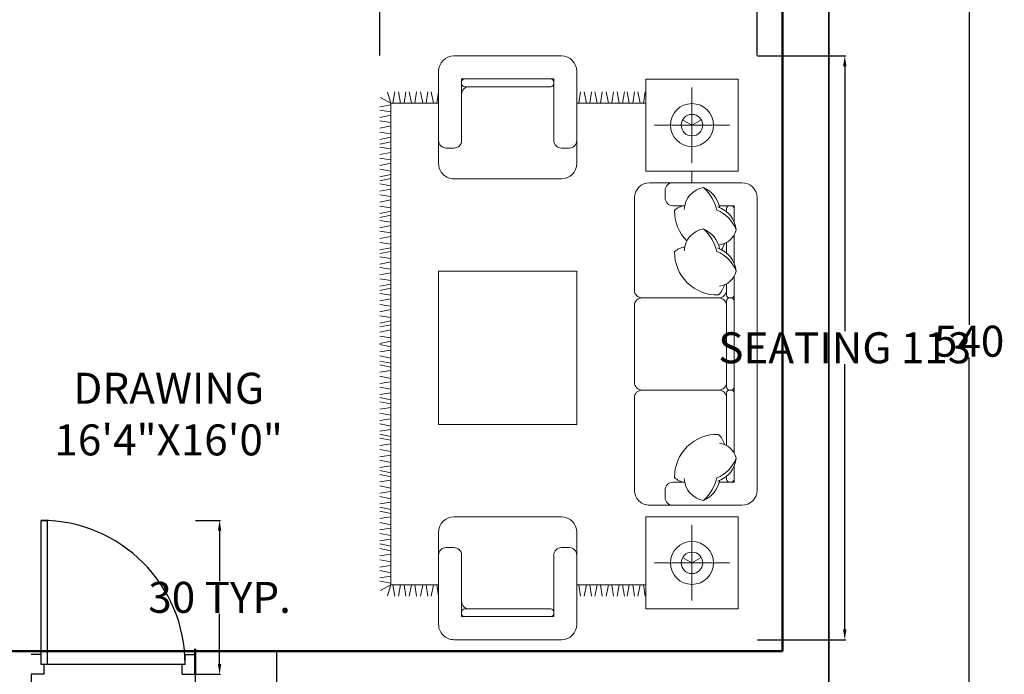
# Model space of a CAD drawing. Units: inches. Extents: x -20 to 10156, y 488 to 2970.
# Tile 4 of 6: x 221 to 412, y 724 to 851. Entities that reach past the tile are written whole.
import ezdxf

# ---------------------------------------------------------------- set-up
doc = ezdxf.new("R2010")
doc.units = ezdxf.units.IN
doc.header["$MEASUREMENT"] = 0
for name, color, linetype, lineweight in [('A-ANNO-DIMS', 2, 'Continuous', 18), ('A-AREA-IDEN', 7, 'Continuous', 25), ('A-DOOR', 4, 'Continuous', 25), ('A-FLOR-STRS', 7, 'Continuous', 25), ('A-FURN', 8, 'Continuous', 18), ('A-WALL', 7, 'Continuous', 50), ('C-PROP', 7, 'Continuous', 35)]:
    doc.layers.add(name, color=color, linetype=linetype, lineweight=lineweight)
doc.styles.get("Standard").update_dxf_attribs({"font": 'arial.ttf'})
doc.dimstyles.get("Standard").update_dxf_attribs({"dimtxt": 6, "dimasz": 2, "dimexe": 0.18, "dimexo": 0.0625, "dimgap": 0.09, "dimtad": 0, "dimtih": 1, "dimtoh": 1, "dimdec": 0, "dimzin": 0, "dimdsep": 46, "dimlunit": 4, "dimtxsty": 'Standard', "dimcen": 0.09, "dimadec": 0, "dimazin": 0, "dimtfac": 1, "dimtdec": 0, "dimtofl": 0, "dimtmove": 0, "dimatfit": 3, "dimfxl": 1, "dimtolj": 1, "dimtzin": 0, "dimarcsym": 0})

# ---------------------------------------------------------------- blocks, each defined once
blk = doc.blocks.new('A$C78AE5658')
for p, q in [((925.1, 3400), (2825.1, 3400)), ((150.1, 3275), (150.1, 2675)), ((750.1, 3275), (150.1, 3275)), ((750.1, 2675), (750.1, 3275)), ((825.1, 2700), (825.1, 3300)), ((2925.1, 3300), (2925.1, 2700)), ((3000.1, 3275), (3000.1, 2675)), ((3600.1, 3275), (3000.1, 3275)), ((3600.1, 2675), (3600.1, 3275)), ((450.1, 2730), (450.1, 3220)), ((975.1, 3250), (975.1, 3151.7)), ((1080.3, 3250), (975.1, 3250)), ((975.1, 3220), (975.1, 3230)), ((995.1, 3250), (1080.3, 3250)), ((1163.5, 3250), (1349.6, 3250)), ((1349.6, 3250), (1163.5, 3250)), ((2586.7, 3250), (1432.8, 3250)), ((1432.8, 3250), (1555.1, 3250)), ((1575.1, 3230), (1575.1, 3220)), ((1575.1, 3220), (1575.1, 3230)), ((1595.1, 3250), (2155.1, 3250)), ((2175.1, 3230), (2175.1, 3220)), ((2175.1, 3230), (2175.1, 3220)), ((2586.7, 3250), (2195.1, 3250)), ((2775.1, 3250), (2669.9, 3250)), ((2755.1, 3250), (2669.9, 3250)), ((2775.1, 3151.7), (2775.1, 3250)), ((2775.1, 3220), (2775.1, 3230)), ((3300.1, 2730), (3300.1, 3220)), ((1013.3, 3200), (995.1, 3200)), ((1282.6, 3200), (1213.8, 3200)), ((1555.1, 3200), (1483.2, 3200)), ((1575.1, 3150), (1575.1, 2650)), ((2155.1, 3200), (1595.1, 3200)), ((2175.1, 3150), (2175.1, 2650)), ((2195.1, 3200), (2536.4, 3200)), ((2737, 3200), (2755.1, 3200)), ((450.1, 2975), (415.1, 3035.6)), ((3300.1, 2975), (3265.1, 3035.6)), ((205.1, 2975), (695.1, 2975)), ((450.1, 2975), (415.1, 2914.4)), ((750.1, 2975), (825.1, 2975)), ((3055.1, 2975), (3545.1, 2975)), ((3300.1, 2975), (3265.1, 2914.4)), ((975.1, 2927.5), (975.1, 2850)), ((2775.1, 2850), (2775.1, 2927.5)), ((925.1, 2800), (875.1, 2800)), ((2875.1, 2800), (2825.1, 2800)), ((150.1, 2675), (750.1, 2675)), ((307.9, 2659.2), (234.4, 2670.3)), ((307.9, 2636.9), (234.4, 2622.4)), ((307.9, 2675), (307.9, 2224.9)), ((3000.1, 2675), (3600.1, 2675)), ((3442.3, 2675), (3442.3, 2224.9)), ((3442.3, 2659.2), (3515.8, 2670.3)), ((3442.3, 2636.9), (3515.8, 2622.4)), ((307.9, 2589), (234.4, 2600.1)), ((307.9, 2566.7), (234.4, 2552.2)), ((1525.1, 2600), (925.1, 2600)), ((2125.1, 2600), (1625.1, 2600)), ((2825.1, 2600), (2225.1, 2600)), ((3442.3, 2589), (3515.8, 2600.1)), ((3442.3, 2566.7), (3515.8, 2552.2)), ((307.9, 2523.5), (234.4, 2534.6)), ((307.9, 2501.3), (234.4, 2486.8)), ((3442.3, 2523.5), (3515.8, 2534.6)), ((3442.3, 2501.3), (3515.8, 2486.8)), ((307.9, 2453.4), (234.4, 2464.5)), ((3442.3, 2453.4), (3515.8, 2464.5)), ((307.9, 2431.1), (234.4, 2416.6)), ((307.9, 2379.6), (234.4, 2390.7)), ((3442.3, 2431.1), (3515.8, 2416.6)), ((3442.3, 2379.6), (3515.8, 2390.7)), ((307.9, 2357.3), (234.4, 2342.8)), ((307.9, 2309.8), (234.4, 2320.9)), ((3442.3, 2357.3), (3515.8, 2342.8)), ((3442.3, 2309.8), (3515.8, 2320.9)), ((307.9, 2287.5), (234.4, 2273)), ((307.9, 2237.8), (234.4, 2248.9)), ((3442.3, 2287.5), (3515.8, 2273)), ((3442.3, 2237.8), (3515.8, 2248.9)), ((100, 2225), (700, 2225)), ((1400.1, 2225), (1400.1, 1325)), ((2400.1, 2225), (1400.1, 2225)), ((2400.1, 1325), (2400.1, 2225)), ((3700.2, 2225), (3100.2, 2225)), ((0, 1425), (0, 2125)), ((600, 2125), (600, 2175)), ((800, 2125), (800, 1425)), ((3000.2, 2125), (3000.2, 1425)), ((3200.2, 2125), (3200.2, 2175)), ((3800.2, 1425), (3800.2, 2125)), ((150, 2075), (150, 1475)), ((550, 2075), (150, 2075)), ((180, 2075), (170, 2075)), ((200, 2036.8), (200, 2055)), ((3250.2, 2075), (3650.2, 2075)), ((3600.2, 2036.8), (3600.2, 2055)), ((3620.2, 2075), (3630.2, 2075)), ((3650.2, 2075), (3650.2, 1475)), ((200, 1495), (200, 2036.8)), ((3600.2, 1495), (3600.2, 2036.8)), ((150, 1886.6), (150, 1495)), ((150, 1886.6), (150, 1475)), ((3650.2, 1886.6), (3650.2, 1495)), ((3650.2, 1886.6), (3650.2, 1475)), ((550, 1475), (150, 1475)), ((150, 1475), (550, 1475)), ((150, 1475), (550, 1475)), ((170, 1475), (180, 1475)), ((170, 1475), (180, 1475)), ((3250.2, 1475), (3650.2, 1475)), ((3650.2, 1475), (3250.2, 1475)), ((3650.2, 1475), (3250.2, 1475)), ((3630.2, 1475), (3620.2, 1475)), ((3630.2, 1475), (3620.2, 1475)), ((600, 1425), (600, 1375)), ((600, 1425), (600, 1375)), ((3200.2, 1425), (3200.2, 1375)), ((3200.2, 1425), (3200.2, 1375)), ((700, 1325), (100, 1325)), ((307.9, 1313.7), (234.4, 1324.8)), ((307.9, 1291.4), (234.4, 1276.9)), ((1400.1, 1325), (2400.1, 1325)), ((3100.2, 1325), (3700.2, 1325)), ((3442.3, 1313.7), (3515.8, 1324.8)), ((3442.3, 1291.4), (3515.8, 1276.9)), ((307.9, 1243.5), (234.4, 1254.6)), ((307.9, 1221.3), (234.4, 1206.8)), ((3442.3, 1243.5), (3515.8, 1254.6)), ((3442.3, 1221.3), (3515.8, 1206.8)), ((307.9, 1169.7), (234.4, 1180.9)), ((3442.3, 1169.7), (3515.8, 1180.9)), ((307.9, 1147.5), (234.4, 1133)), ((307.9, 1099.9), (234.4, 1111.1)), ((3442.3, 1147.5), (3515.8, 1133)), ((3442.3, 1099.9), (3515.8, 1111.1)), ((307.9, 1077.7), (234.4, 1063.2)), ((307.9, 1028), (234.4, 1039.1)), ((3442.3, 1077.7), (3515.8, 1063.2)), ((3442.3, 1028), (3515.8, 1039.1)), ((307.9, 1015), (235.6, 991.4)), ((307.9, 1015), (270, 945.8)), ((317.2, 1015), (331.8, 941.5)), ((363.4, 1015), (352.3, 941.5)), ((385.6, 1015), (400.1, 941.5)), ((433.5, 1015), (422.4, 941.5)), ((455.8, 1015), (470.3, 941.5)), ((507.3, 1015), (496.2, 941.5)), ((529.5, 1015), (544.1, 941.5)), ((559.2, 1015), (573.7, 941.5)), ((605.3, 1015), (594.2, 941.5)), ((627.6, 1015), (642.1, 941.5)), ((675.5, 1015), (664.4, 941.5)), ((697.7, 1015), (712.2, 941.5)), ((749.3, 1015), (738.1, 941.5)), ((771.5, 1015), (786, 941.5)), ((798.4, 1015), (813, 941.5)), ((844.6, 1015), (833.5, 941.5)), ((866.8, 1015), (881.3, 941.5)), ((914.7, 1015), (903.6, 941.5)), ((937, 1015), (951.5, 941.5)), ((988.5, 1015), (977.4, 941.5)), ((1010.7, 1015), (1025.3, 941.5)), ((1036.1, 1015), (1050.6, 941.5)), ((1082.2, 1015), (1071.1, 941.5)), ((1104.4, 1015), (1119, 941.5)), ((1152.4, 1015), (1141.3, 941.5)), ((1174.6, 1015), (1189.1, 941.5)), ((1226.1, 1015), (1215, 941.5)), ((1248.4, 1015), (1262.9, 941.5)), ((1272.6, 1015), (1287.1, 941.5)), ((1318.7, 1015), (1307.6, 941.5)), ((1341, 1015), (1355.5, 941.5)), ((1388.9, 1015), (1377.8, 941.5)), ((1411.1, 1015), (1425.6, 941.5)), ((1462.7, 1015), (1451.5, 941.5)), ((1484.9, 1015), (1499.4, 941.5)), ((1511.9, 1015), (1526.4, 941.5)), ((1558, 1015), (1546.9, 941.5)), ((1580.2, 1015), (1594.7, 941.5)), ((1628.1, 1015), (1617, 941.5)), ((1650.4, 1015), (1664.9, 941.5)), ((1701.9, 1015), (1690.8, 941.5)), ((1724.2, 1015), (1738.7, 941.5)), ((1749.7, 1015), (1764.3, 941.5)), ((1782.8, 1015), (1797.3, 941.5)), ((1834.3, 1015), (1823.2, 941.5)), ((1856.6, 1015), (1871.1, 941.5)), ((1893.7, 1015), (1879.1, 941.5)), ((1915.9, 1015), (1927, 941.5)), ((1967.4, 1015), (1952.9, 941.5)), ((2000.5, 1015), (1986, 941.5)), ((2026.1, 1015), (2011.6, 941.5)), ((2048.3, 1015), (2059.4, 941.5)), ((2099.8, 1015), (2085.3, 941.5)), ((2122.1, 1015), (2133.2, 941.5)), ((2170, 1015), (2155.5, 941.5)), ((2192.2, 1015), (2203.4, 941.5)), ((2238.4, 1015), (2223.9, 941.5)), ((2265.3, 1015), (2250.8, 941.5)), ((2287.6, 1015), (2298.7, 941.5)), ((2339.1, 1015), (2324.6, 941.5)), ((2361.3, 1015), (2372.4, 941.5)), ((2409.2, 1015), (2394.7, 941.5)), ((2431.5, 1015), (2442.6, 941.5)), ((2477.6, 1015), (2463.1, 941.5)), ((2501.8, 1015), (2487.3, 941.5)), ((2524.1, 1015), (2535.2, 941.5)), ((2575.6, 1015), (2561.1, 941.5)), ((2597.9, 1015), (2609, 941.5)), ((2645.8, 1015), (2631.3, 941.5)), ((2668, 1015), (2679.1, 941.5)), ((2714.1, 1015), (2699.6, 941.5)), ((2739.5, 1015), (2725, 941.5)), ((2761.7, 1015), (2772.8, 941.5)), ((2813.2, 1015), (2798.7, 941.5)), ((2835.5, 1015), (2846.6, 941.5)), ((2883.4, 1015), (2868.9, 941.5)), ((2905.7, 1015), (2916.8, 941.5)), ((2951.8, 1015), (2937.3, 941.5)), ((2978.7, 1015), (2964.2, 941.5)), ((3001, 1015), (3012.1, 941.5)), ((3052.5, 1015), (3038, 941.5)), ((3074.7, 1015), (3085.8, 941.5)), ((3122.7, 1015), (3108.1, 941.5)), ((3144.9, 1015), (3156, 941.5)), ((3191, 1015), (3176.5, 941.5)), ((3220.7, 1015), (3206.2, 941.5)), ((3242.9, 1015), (3254, 941.5)), ((3294.4, 1015), (3279.9, 941.5)), ((3316.7, 1015), (3327.8, 941.5)), ((3364.6, 1015), (3350.1, 941.5)), ((3386.9, 1015), (3398, 941.5)), ((3433, 1015), (3418.5, 941.5)), ((3442.3, 1015), (3514.7, 991.4)), ((3442.3, 1015), (3480.2, 945.8))]:
    blk.add_line(p, q)
for points in [[(307.9, 1325), (307.9, 1015), (1875.1, 1015)], [(3442.3, 1325), (3442.3, 1015), (1875.1, 1015)]]:
    blk.add_lwpolyline(points)
for centre, radius in [((450.1, 2975), 140), ((3300.1, 2975), 140), ((450.1, 2975), 70), ((3300.1, 2975), 70)]:
    blk.add_circle(centre, radius)
for centre, radius, start, end in [((925.1, 3300), 100, 90, 180), ((2825.1, 3300), 100, 0, 90), ((995.1, 3230), 20, 90, 180), ((995.1, 3220), 20, 180, 270), ((1145.5, 3092.7), 170.3, 94.53318, 162.72864), ((1208.5, 3055.2), 220.9, 110.25938, 158.43175), ((1100.2, 3136), 130.4, 7.76802, 75.89361), ((1414.8, 3092.7), 170.3, 94.53318, 162.72864), ((1477.9, 3055.2), 220.9, 110.25938, 158.43175), ((1369.6, 3136), 130.4, 7.76802, 75.89361), ((1555.1, 3230), 20, 0, 90), ((1555.1, 3220), 20, 270, 0), ((1595.1, 3230), 20, 90, 180), ((1595.1, 3220), 20, 180, 270), ((2155.1, 3230), 20, 0, 90), ((2155.1, 3220), 20, 270, 0), ((2195.1, 3230), 20, 90, 180), ((2195.1, 3220), 20, 180, 270), ((2650, 3136), 130.4, 104.10639, 172.23198), ((2541.7, 3055.2), 220.9, 21.56825, 69.74062), ((2604.8, 3092.7), 170.3, 17.27136, 85.46682), ((2755.1, 3230), 20, 0, 90), ((2755.1, 3220), 20, 270, 0), ((1019.4, 2980.4), 176.9, 100.63867, 156.68485), ((1288.8, 2980.4), 176.9, 100.63867, 156.68485), ((1173.4, 3032.5), 161.7, 56.77866, 73.22072), ((1278.1, 3139.5), 278.1, 269.42107, 1.71498), ((1442.7, 3032.5), 161.7, 45.50553, 73.22072), ((1525.1, 3150), 50, 0, 90), ((1625.1, 3150), 50, 90, 180), ((2125.1, 3150), 50, 0, 90), ((2225.1, 3150), 50, 90, 180), ((2741.5, 3139.5), 278.1, 178.28502, 270.57893), ((2576.8, 3032.5), 161.7, 106.77928, 134.49447), ((2730.8, 2980.4), 176.9, 23.31515, 79.36133), ((1072.2, 2851.5), 293.1, 103.64916, 137.26323), ((1341.6, 2851.5), 293.1, 103.64916, 137.26323), ((2678, 2851.5), 293.1, 42.73677, 76.35084), ((1005.6, 3075.1), 150.7, 189.39285, 267.93283), ((1275, 3075.1), 150.7, 189.39285, 267.93283), ((2744.6, 3075.1), 150.7, 272.06717, 350.60715), ((1087.5, 2939.9), 113.2, 186.29025, 223.8884), ((1008.7, 3139.5), 278.1, 269.42107, 314.71173), ((1356.9, 2939.9), 113.2, 186.29025, 223.8884), ((2662.7, 2939.9), 113.2, 316.1116, 353.70975), ((875.1, 2850), 50, 180, 270), ((925.1, 2850), 50, 270, 0), ((2825.1, 2850), 50, 180, 270), ((2875.1, 2850), 50, 270, 0), ((925.1, 2700), 100, 180, 270), ((2825.1, 2700), 100, 270, 0), ((1525.1, 2650), 50, 270, 0), ((1625.1, 2650), 50, 180, 270), ((2125.1, 2650), 50, 270, 0), ((2225.1, 2650), 50, 180, 270), ((100, 2125), 100, 90, 180), ((550, 2175), 50, 0, 90), ((700, 2125), 100, 0, 90), ((3100.2, 2125), 100, 90, 180), ((3250.2, 2175), 50, 90, 180), ((3700.2, 2125), 100, 0, 90), ((550, 2125), 50, 270, 0), ((3250.2, 2125), 50, 180, 270), ((170, 2055), 20, 90, 180), ((180, 2055), 20, 0, 90), ((3620.2, 2055), 20, 90, 180), ((3630.2, 2055), 20, 0, 90), ((170, 1495), 20, 180, 270), ((180, 1495), 20, 270, 0), ((250, 1525), 50, 180, 270), ((550, 1425), 50, 0, 90), ((550, 1425), 50, 0, 90), ((3250.2, 1425), 50, 90, 180), ((3250.2, 1425), 50, 90, 180), ((3550.2, 1525), 50, 270, 0), ((3620.2, 1495), 20, 180, 270), ((3630.2, 1495), 20, 270, 0), ((100, 1425), 100, 180, 270), ((700, 1425), 100, 270, 0), ((3100.2, 1425), 100, 180, 270), ((3700.2, 1425), 100, 270, 0), ((550, 1375), 50, 270, 0), ((550, 1375), 50, 270, 0), ((3250.2, 1375), 50, 180, 270), ((3250.2, 1375), 50, 180, 270)]:
    blk.add_arc(centre, radius, start, end)
blk = doc.blocks.new('A$C72DF01B0')
for p, q in [((50, 100), (0, 100)), ((780, 50), (780, 100)), ((780, 100), (830, 100)), ((65, 0), (65, 50)), ((780, 50), (80, 50)), ((765, 0), (765, 50)), ((65, 0), (0, 0)), ((765, 0), (830, 0))]:
    blk.add_line(p, q)
blk.add_lwpolyline([(50, 780), (80, 780), (80, 50), (50, 50)], close=True)
blk.add_arc((50, 50), 730, 0, 90)
blk = doc.blocks.new('*D12')
at = {"layer": 'A-ANNO-DIMS', "color": 0, "lineweight": -2, "transparency": 16777216}
for p, q in [((223.3, 724.17), (223.3, 719.29)), ((255.01, 724.17), (255.01, 719.29)), ((225.3, 719.47), (253.01, 719.47)), ((255.01, 719.47), (257.01, 719.47))]:
    blk.add_line(p, q, dxfattribs=at)
at = {"layer": 'A-ANNO-DIMS', "color": 0, "transparency": 16777216}
for points in [[(225.3, 719.81), (225.3, 719.14), (223.3, 719.47)], [(253.01, 719.81), (253.01, 719.14), (255.01, 719.47)]]:
    blk.add_solid(points, dxfattribs=at)
at = {"layer": 'Defpoints', "color": 0, "transparency": 16777216}
for p in [(223.3, 724.23), (255.01, 724.23), (255.01, 719.47)]:
    blk.add_point(p, dxfattribs=at)
at = {"layer": 'A-ANNO-DIMS', "color": 0, "transparency": 16777216, "insert": (285.29, 719.47), "char_height": 6, "attachment_point": 5}
blk.add_mtext('\\A1;DOOR 32 TYP.', dxfattribs=at)
blk = doc.blocks.new('*D13')
at = {"layer": 'A-ANNO-DIMS', "color": 0, "lineweight": -2, "transparency": 16777216}
for p, q in [((255.07, 754.03), (259.95, 754.03)), ((259.77, 752.03), (259.77, 742.29)), ((259.77, 726.23), (259.77, 735.97)), ((255.07, 724.23), (259.95, 724.23))]:
    blk.add_line(p, q, dxfattribs=at)
at = {"layer": 'A-ANNO-DIMS', "color": 0, "transparency": 16777216}
for points in [[(259.43, 752.03), (260.1, 752.03), (259.77, 754.03)], [(259.43, 726.23), (260.1, 726.23), (259.77, 724.23)]]:
    blk.add_solid(points, dxfattribs=at)
at = {"layer": 'Defpoints', "color": 0, "transparency": 16777216}
for p in [(255.01, 754.03), (259.77, 754.03), (255.01, 724.23)]:
    blk.add_point(p, dxfattribs=at)
at = {"layer": 'A-ANNO-DIMS', "color": 0, "transparency": 16777216, "insert": (259.77, 739.13), "char_height": 6, "attachment_point": 5}
blk.add_mtext('\\A1;30 TYP.', dxfattribs=at)
blk = doc.blocks.new('*D22')
at = {"layer": 'A-ANNO-DIMS', "color": 0, "lineweight": -2, "transparency": 16777216}
for p, q in [((363.97, 843.96), (381.04, 843.96)), ((380.86, 841.96), (380.86, 790.64)), ((380.86, 732.93), (380.86, 784.25)), ((363.97, 730.93), (381.04, 730.93))]:
    blk.add_line(p, q, dxfattribs=at)
at = {"layer": 'A-ANNO-DIMS', "color": 0, "transparency": 16777216}
for points in [[(380.53, 841.96), (381.2, 841.96), (380.86, 843.96)], [(380.53, 732.93), (381.2, 732.93), (380.86, 730.93)]]:
    blk.add_solid(points, dxfattribs=at)
at = {"layer": 'Defpoints', "color": 0, "transparency": 16777216}
for p in [(363.91, 843.96), (363.91, 730.93), (380.86, 730.93)]:
    blk.add_point(p, dxfattribs=at)
at = {"layer": 'A-ANNO-DIMS', "color": 0, "transparency": 16777216, "insert": (380.86, 787.45), "char_height": 6, "attachment_point": 5}
blk.add_mtext('\\A1;SEATING 113', dxfattribs=at)
blk = doc.blocks.new('*D23')
at = {"layer": 'A-ANNO-DIMS', "color": 0, "lineweight": -2, "transparency": 16777216}
for p, q in [((290.79, 844.02), (290.79, 861.1)), ((292.79, 860.92), (322.98, 860.92)), ((361.91, 860.92), (331.71, 860.92)), ((363.91, 844.02), (363.91, 861.1))]:
    blk.add_line(p, q, dxfattribs=at)
at = {"layer": 'A-ANNO-DIMS', "color": 0, "transparency": 16777216}
for points in [[(292.79, 861.25), (292.79, 860.58), (290.79, 860.92)], [(361.91, 861.25), (361.91, 860.58), (363.91, 860.92)]]:
    blk.add_solid(points, dxfattribs=at)
at = {"layer": 'Defpoints', "color": 0, "transparency": 16777216}
for p in [(363.91, 860.92), (290.79, 843.96), (363.91, 843.96)]:
    blk.add_point(p, dxfattribs=at)
at = {"layer": 'A-ANNO-DIMS', "color": 0, "transparency": 16777216, "insert": (327.35, 860.92), "char_height": 6, "attachment_point": 5}
blk.add_mtext('\\A1;73', dxfattribs=at)
blk = doc.blocks.new('*D29')
at = {"layer": 'A-ANNO-DIMS', "color": 0, "lineweight": -2, "transparency": 16777216}
for p, q in [((377.86, 1058.73), (405.13, 1058.73)), ((404.95, 1056.73), (404.95, 791.88)), ((404.95, 520.73), (404.95, 785.58)), ((377.86, 518.73), (405.13, 518.73))]:
    blk.add_line(p, q, dxfattribs=at)
at = {"layer": 'A-ANNO-DIMS', "color": 0, "transparency": 16777216}
for points in [[(404.62, 1056.73), (405.28, 1056.73), (404.95, 1058.73)], [(404.62, 520.73), (405.28, 520.73), (404.95, 518.73)]]:
    blk.add_solid(points, dxfattribs=at)
at = {"layer": 'Defpoints', "color": 0, "transparency": 16777216}
for p in [(377.8, 1058.73), (404.95, 1058.73), (377.8, 518.73)]:
    blk.add_point(p, dxfattribs=at)
at = {"layer": 'A-ANNO-DIMS', "color": 0, "transparency": 16777216, "insert": (404.95, 788.73), "char_height": 6, "attachment_point": 5}
blk.add_mtext('\\A1;540', dxfattribs=at)

msp = doc.modelspace()

# ---------------------------------------------------------------- linework, layer by layer
at = {"layer": 'A-FLOR-STRS'}
msp.add_line((270.8, 728.73), (270.8, 686.23), dxfattribs=at)
at = {"layer": 'A-WALL'}
for p, q in [((368.8, 917.23), (368.8, 728.73)), ((218.8, 728.73), (368.8, 728.73)), ((255.01, 724.23), (255.01, 729.15))]:
    msp.add_line(p, q, dxfattribs=at)
at = {"layer": 'C-PROP'}
msp.add_line((377.8, 1058.73), (377.8, 518.73), dxfattribs=at)

# ---------------------------------------------------------------- block references
at = {"layer": 'A-DOOR', "xscale": 0.0382046374882532, "yscale": 0.0382046374882532, "zscale": 0.0382046374882532}
msp.add_blockref('A$C72DF01B0', (223.3, 724.23), dxfattribs=at)
at = {"layer": 'A-FURN', "xscale": 0.0297428240468277, "yscale": 0.0297428240468277, "zscale": 0.0297428240468277, "rotation": 270}
msp.add_blockref('A$C78AE5658', (262.78, 843.96), dxfattribs=at)

# ---------------------------------------------------------------- texts
at = {"layer": 'A-AREA-IDEN', "insert": (192.92, 782.62), "char_height": 6, "attachment_point": 1}
msp.add_mtext_dynamic_manual_height_columns('\\pxqc;DRAWING\\P16\'4"X16\'0"', width=113.9748, gutter_width=30, heights=[0], dxfattribs=at)

# ---------------------------------------------------------------- dimensions: what is measured, and where the dimension line sits
at = {"layer": 'A-ANNO-DIMS'}
dim = msp.add_linear_dim(base=(404.95, 1058.73), p1=(377.8, 518.73), p2=(377.8, 1058.73), angle=90, dimstyle='Standard', override={"dimdec": 0, "dimlfac": 1, "dimrnd": 0, "dimzin": 0, "dimdsep": 46, "dimlunit": 2}, dxfattribs=at)
dim.commit()
dim.dimension.update_dxf_attribs({"geometry": '*D29', "text_midpoint": (404.95, 788.73)})
dim = msp.add_linear_dim(base=(363.91, 860.92), p1=(290.79, 843.96), p2=(363.91, 843.96), dimstyle='Standard', override={"dimdec": 0, "dimlfac": 1, "dimrnd": 0, "dimzin": 0, "dimdsep": 46, "dimlunit": 2}, dxfattribs=at)
dim.commit()
dim.dimension.update_dxf_attribs({"geometry": '*D23', "text_midpoint": (327.35, 860.92)})
for base, p1, p2, angle, text, picture, middle in [((380.86, 730.93), (363.91, 843.96), (363.91, 730.93), 270, 'SEATING <>', '*D22', (380.86, 787.45)), ((259.77, 754.03), (255.01, 724.23), (255.01, 754.03), 90, '<> TYP.', '*D13', (259.77, 739.13))]:
    dim = msp.add_linear_dim(base=base, p1=p1, p2=p2, angle=angle, text=text, dimstyle='Standard', override={"dimdec": 0, "dimlfac": 1, "dimrnd": 0, "dimzin": 0, "dimdsep": 46, "dimlunit": 2}, dxfattribs=at)
    dim.commit()
    dim.dimension.update_dxf_attribs({"geometry": picture, "text_midpoint": middle})
dim = msp.add_linear_dim(base=(255.01, 719.47), p1=(223.3, 724.23), p2=(255.01, 724.23), text='DOOR <> TYP.', dimstyle='Standard', override={"dimdec": 0, "dimlfac": 1, "dimrnd": 0, "dimzin": 0, "dimdsep": 46, "dimlunit": 2}, dxfattribs=at)
dim.commit()
dim.dimension.update_dxf_attribs({"geometry": '*D12', "text_midpoint": (285.29, 719.47)})

doc.saveas('drawing.dxf')
